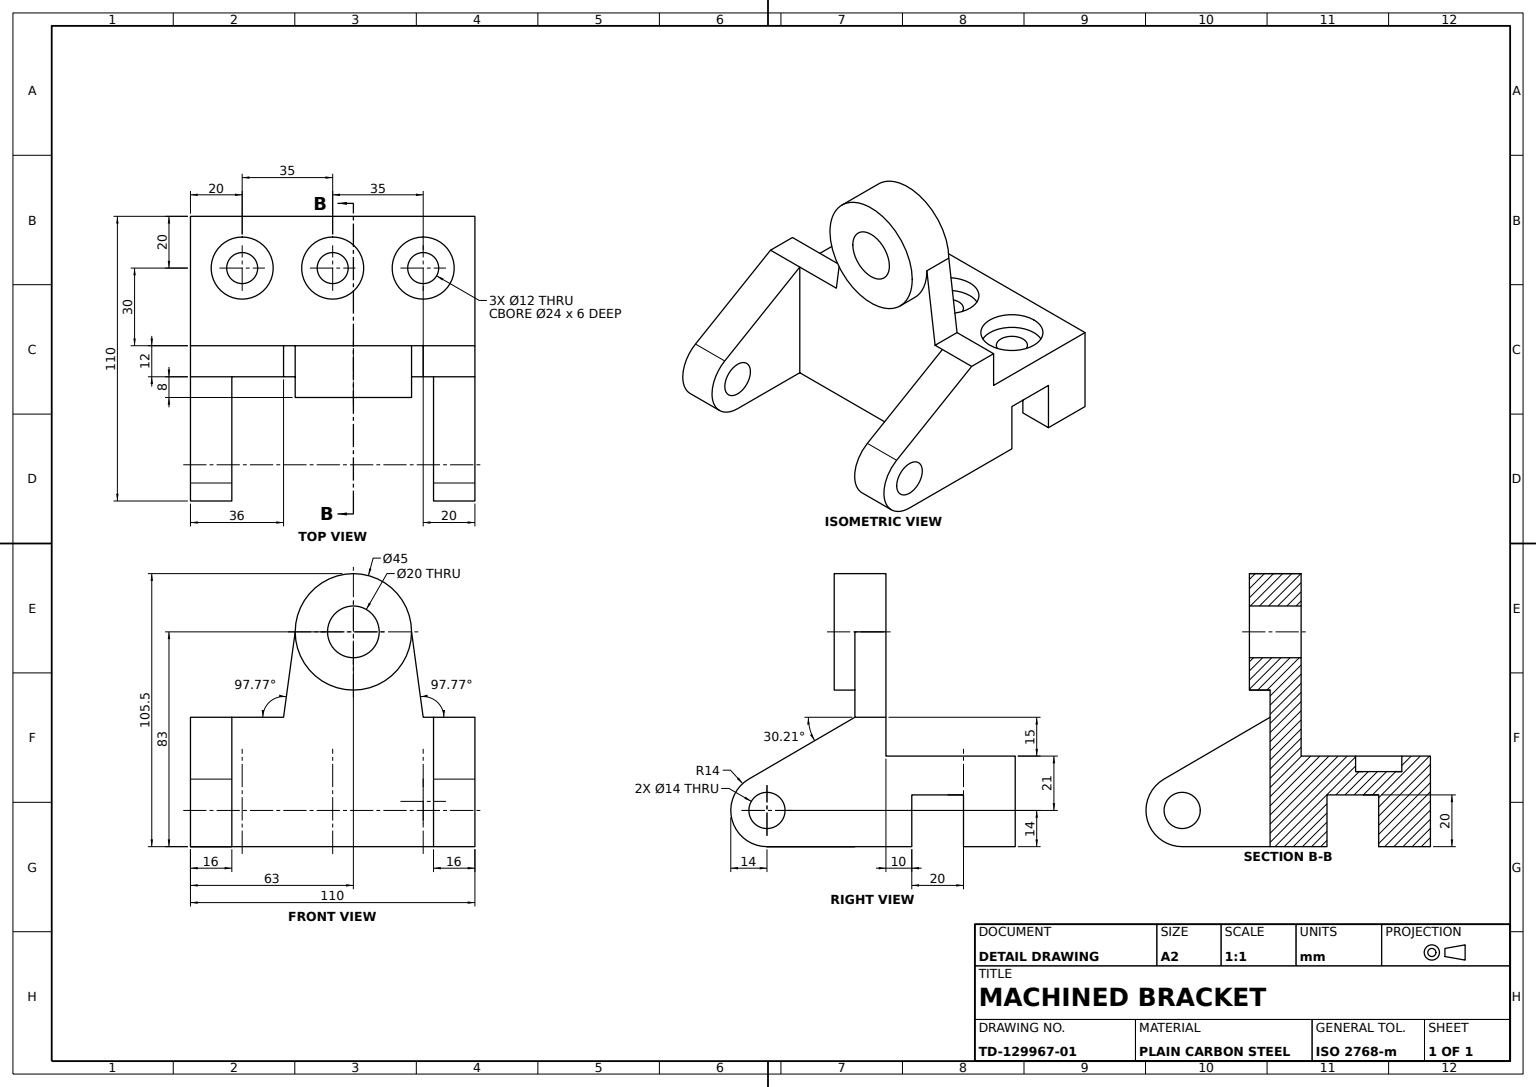
SolidWorks part; units mm, degrees
material "Plain Carbon Steel"
ref_plane "Front Plane" through (0, 0, 0) normal (0, 0, 1) x (1, 0, 0)
ref_plane "Top Plane" through (0, 0, 0) normal (0, 1, 0) x (1, 0, 0)
ref_plane "Right Plane" through (0, 0, 0) normal (1, 0, 0) x (0, 0, -1)
sketch "Side Arm Profile" plane through (0, 0, 0) normal (1, 0, 0) x (0, 0, -1)
  line L0 (0, 0) -> (-20, 0)
  line L1 (-20, 0) -> (-20, 20)
  line L2 (-20, 20) -> (-40, 20)
  line L3 (-40, 20) -> (-40, 0)
  line L4 (-40, 0) -> (-96, 0)
  line L6 (0, 0) -> (0, 35)
  line L7 (0, 35) -> (-50, 35)
  line L8 (-50, 35) -> (-50, 50)
  line L9 (-50, 50) -> (-62, 50)
  line L10 (-62, 50) -> (-103.0451, 26.0982)
  arc A0 (-103.0451, 26.0982) -> (-96, 0) centre (-96, 14) ccw
  point P8 (-30, 20)
  dimension "D8" = 14
  dimension "D1" = 56
  dimension "D2" = 20
  dimension "D3" = 20
  dimension "D4" = 35
  dimension "D5" = 15
  dimension "D6" = 12
  dimension "D7" = 47.4974
  dimension "D9" = 20
extrude "Side Arm 16mm" add sketch "Side Arm Profile" against normal blind 16
sketch "Bracket Body Profile" plane through (-16, 0, 0) normal (-1, 0, 0) x (0, 0, 1)
  line L0 (0, 0) -> (0, 35)
  line L1 (0, 35) -> (50, 35)
  line L2 (50, 35) -> (50, 50)
  line L3 (50, 50) -> (62, 50)
  line L4 (62, 50) -> (62, 0)
  line L5 (96, 0) -> (40, 0) construction
  line L6 (62, 0) -> (40, 0)
  line L7 (40, 0) -> (40, 20)
  line L8 (40, 20) -> (20, 20)
  line L9 (20, 20) -> (20, 0)
  line L10 (20, 0) -> (0, 0)
extrude "Bracket Body 94mm" add sketch "Bracket Body Profile" along normal blind 94
sketch "Second Arm Profile" plane through (-110, 0, 0) normal (-1, 0, 0) x (0, 0, 1)
  line L0 (62, 0) -> (62, 50)
  line L1 (62, 50) -> (103.0451, 26.0982)
  line L2 (62, 0) -> (96, 0)
  arc A0 (96, 0) -> (103.0451, 26.0982) centre (96, 14) ccw
extrude "Second Arm 16mm" add sketch "Second Arm Profile" against normal blind 16
sketch "Pivot Hole Sketch Ø14" plane through (0, 0, 0) normal (1, 0, 0) x (0, 0, -1)
  circle A0 centre (-96, 14) radius 7
  dimension "D1" = 14
extrude "Pivot Holes Ø14 Through" cut sketch "Pivot Hole Sketch Ø14" against normal blind 231
sketch "Bearing Boss Sketch Ø45" plane through (0, 0, 62) normal (0, 0, 1) x (1, 0, 0)
  line L0 (-94, 0) -> (-16, 0) construction
  line L2 (0, 0) -> (0, 26.0982) construction
  circle A0 centre (-47, 83) radius 22.5
  dimension "D1" = 45
  dimension "D2" = 83
  dimension "D3" = 47
extrude "Bearing Boss Ø45" add sketch "Bearing Boss Sketch Ø45" along normal blind 8 and the other way blind 12 separate body
sketch "Boss Support Web Profile" plane through (0, 0, 62) normal (0, 0, 1) x (1, 0, 0)
  line L1 (-94, 50) -> (-16, 50) construction
  line L2 (-20, 50) -> (-24.5, 83)
  line L3 (-94, 50) -> (-94, 0) construction
  line L4 (-74, 50) -> (-69.5, 83)
  line L5 (-74, 50) -> (-20, 50)
  circle A0 centre (-47, 83) radius 22.5 construction
  arc A1 (-69.5, 83) -> (-24.5, 83) centre (-47, 83) ccw
  dimension "D1" = 33
  dimension "D2" = 33
  dimension "D3" = 80.0771
  dimension "D4" = 7.765
extrude "Boss Support Web 12mm" add sketch "Boss Support Web Profile" against normal blind 12
sketch "Bearing Bore Sketch Ø20" plane through (0, 0, 70) normal (0, 0, 1) x (1, 0, 0)
  circle A0 centre (-47, 83) radius 10
  dimension "D1" = 20
extrude "Bearing Bore Ø20" cut sketch "Bearing Bore Sketch Ø20" against normal blind 101
sketch "Counterbore Sketch Ø24" plane through (0, 35, 0) normal (0, 1, 0) x (1, 0, 0)
  line L0 (-110, -50) -> (-110, 0) construction
  line L1 (0, 0) -> (0, -50) construction
  circle A0 centre (-20, -20) radius 12
  circle A1 centre (-55, -20) radius 12
  circle A2 centre (-90, -20) radius 12
  dimension "D1" = 24
  dimension "D2" = 20
  dimension "D6" = 24
  dimension "D7" = 24
  dimension "D8" = 28.2843
  dimension "D3" = 35
  dimension "D4" = 35
  dimension "D5" = 20
extrude "Counterbores Ø24x6" cut sketch "Counterbore Sketch Ø24" against normal blind 6
sketch "Mounting Hole Sketch Ø12" plane through (0, 29, 0) normal (0, 1, 0) x (1, 0, 0)
  circle A0 centre (-20, -20) radius 6
  circle A1 centre (-55, -20) radius 6
  circle A2 centre (-90, -20) radius 6
  dimension "D1" = 12
  dimension "D2" = 12
  dimension "D3" = 12
extrude "Mounting Holes Ø12" cut sketch "Mounting Hole Sketch Ø12" against normal blind 58
